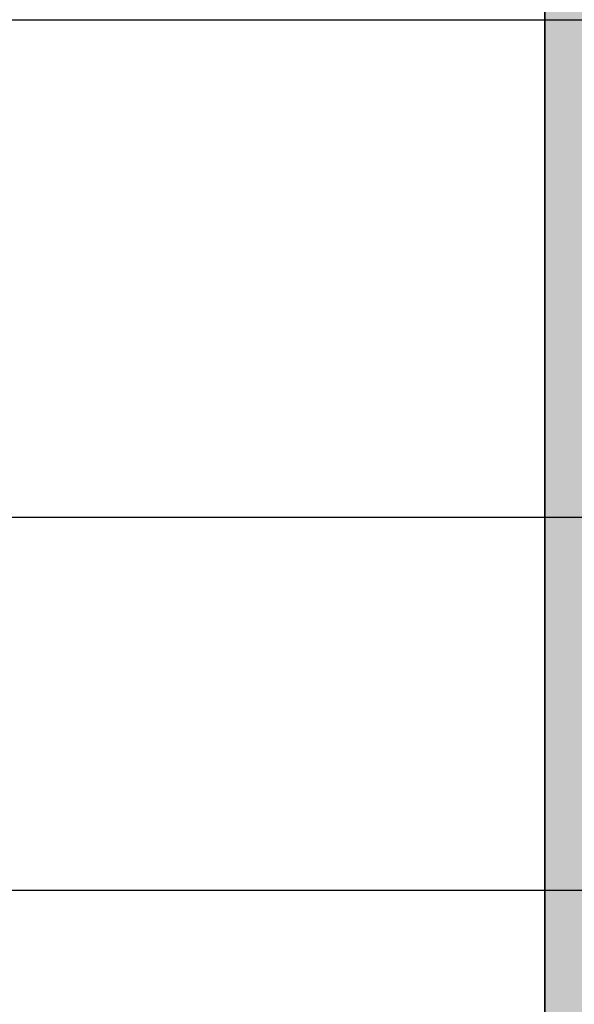
# Model space of a CAD drawing. Units: inches. Extents: x 925 to 2834, y 111 to 1355.
# Tile 20 of 25: x 1737 to 1844, y 882 to 1072. Entities that reach past the tile are written whole.
import ezdxf

# ---------------------------------------------------------------- set-up
doc = ezdxf.new("R2010")
doc.units = ezdxf.units.IN
doc.header["$MEASUREMENT"] = 0
for name, color, linetype, lineweight in [('A-ANNO-DIMS', 2, 'Continuous', 18), ('A-ANNO-TTLB', 7, 'Continuous', 35), ('A-FLOR-PATT', 252, 'Continuous', 13)]:
    doc.layers.add(name, color=color, linetype=linetype, lineweight=lineweight)
doc.styles.get("Standard").update_dxf_attribs({"font": 'arial.ttf'})
doc.dimstyles.get("Standard").update_dxf_attribs({"dimtxt": 6, "dimasz": 3, "dimexe": 0.18, "dimexo": 0.0625, "dimgap": 0.09, "dimtad": 0, "dimtih": 1, "dimtoh": 1, "dimdec": 1, "dimzin": 0, "dimdsep": 46, "dimlunit": 3, "dimtxsty": 'Standard', "dimblk": 'ARCHTICK', "dimcen": 0.09, "dimadec": 0, "dimazin": 0, "dimtfac": 1, "dimtdec": 1, "dimtofl": 0, "dimtmove": 0, "dimatfit": 3, "dimfxl": 1, "dimtolj": 1, "dimtzin": 0, "dimarcsym": 0})

# ---------------------------------------------------------------- blocks, each defined once
blk = doc.blocks.new('_ArchTick')
at = {"color": 0, "linetype": 'ByBlock', "const_width": 0.15}
blk.add_lwpolyline([(-0.5, -0.5), (0.5, 0.5)], dxfattribs=at)
blk = doc.blocks.new('*D47')
at = {"layer": 'A-ANNO-DIMS', "color": 0, "lineweight": -2, "transparency": 16777216}
for p, q in [((1708.78, 903.59), (1988.62, 903.59)), ((1988.44, 903.59), (1988.44, 869.23)), ((1988.44, 828.59), (1988.44, 862.95)), ((1708.78, 828.59), (1988.62, 828.59))]:
    blk.add_line(p, q, dxfattribs=at)
at = {"layer": 'Defpoints', "color": 0, "transparency": 16777216}
for p in [(1708.71, 903.59), (1988.44, 903.59), (1708.71, 828.59)]:
    blk.add_point(p, dxfattribs=at)
at = {"layer": 'A-ANNO-DIMS', "color": 0, "lineweight": -2, "transparency": 16777216, "xscale": 3, "yscale": 3, "zscale": 3}
for p, rotation in [((1988.44, 903.59), 90), ((1988.44, 828.59), 270)]:
    blk.add_blockref('_ArchTick', p, dxfattribs=dict(at, rotation=rotation))
at = {"layer": 'A-ANNO-DIMS', "color": 0, "transparency": 16777216, "insert": (1988.44, 866.09), "char_height": 6, "attachment_point": 5}
blk.add_mtext('\\A1;75', dxfattribs=at)
blk = doc.blocks.new('*D48')
at = {"layer": 'A-ANNO-DIMS', "color": 0, "lineweight": -2, "transparency": 16777216}
for p, q in [((1708.78, 975.59), (1988.62, 975.59)), ((1988.44, 975.59), (1988.44, 942.69)), ((1988.44, 903.59), (1988.44, 936.49)), ((1708.78, 903.59), (1988.62, 903.59))]:
    blk.add_line(p, q, dxfattribs=at)
at = {"layer": 'Defpoints', "color": 0, "transparency": 16777216}
for p in [(1708.71, 975.59), (1988.44, 975.59), (1708.71, 903.59)]:
    blk.add_point(p, dxfattribs=at)
at = {"layer": 'A-ANNO-DIMS', "color": 0, "lineweight": -2, "transparency": 16777216, "xscale": 3, "yscale": 3, "zscale": 3}
for p, rotation in [((1988.44, 975.59), 90), ((1988.44, 903.59), 270)]:
    blk.add_blockref('_ArchTick', p, dxfattribs=dict(at, rotation=rotation))
at = {"layer": 'A-ANNO-DIMS', "color": 0, "transparency": 16777216, "insert": (1988.44, 939.59), "char_height": 6, "attachment_point": 5}
blk.add_mtext('\\A1;72', dxfattribs=at)
blk = doc.blocks.new('*D49')
at = {"layer": 'A-ANNO-DIMS', "color": 0, "lineweight": -2, "transparency": 16777216}
for p, q in [((1708.78, 1071.59), (1988.62, 1071.59)), ((1988.44, 1071.59), (1988.44, 1026.74)), ((1988.44, 975.59), (1988.44, 1020.44)), ((1708.78, 975.59), (1988.62, 975.59))]:
    blk.add_line(p, q, dxfattribs=at)
at = {"layer": 'Defpoints', "color": 0, "transparency": 16777216}
for p in [(1708.71, 1071.59), (1988.44, 1071.59), (1708.71, 975.59)]:
    blk.add_point(p, dxfattribs=at)
at = {"layer": 'A-ANNO-DIMS', "color": 0, "lineweight": -2, "transparency": 16777216, "xscale": 3, "yscale": 3, "zscale": 3}
for p, rotation in [((1988.44, 1071.59), 90), ((1988.44, 975.59), 270)]:
    blk.add_blockref('_ArchTick', p, dxfattribs=dict(at, rotation=rotation))
at = {"layer": 'A-ANNO-DIMS', "color": 0, "transparency": 16777216, "insert": (1988.44, 1023.59), "char_height": 6, "attachment_point": 5}
blk.add_mtext('\\A1;96', dxfattribs=at)
blk = doc.blocks.new('*D50')
at = {"layer": 'A-ANNO-DIMS', "color": 0, "lineweight": -2, "transparency": 16777216}
for p, q in [((1718.78, 1081.59), (1988.62, 1081.59)), ((1988.44, 1081.59), (1988.44, 1079.74)), ((1988.44, 1071.59), (1988.44, 1073.44)), ((1708.78, 1071.59), (1988.62, 1071.59))]:
    blk.add_line(p, q, dxfattribs=at)
at = {"layer": 'Defpoints', "color": 0, "transparency": 16777216}
for p in [(1718.71, 1081.59), (1988.44, 1081.59), (1708.71, 1071.59)]:
    blk.add_point(p, dxfattribs=at)
at = {"layer": 'A-ANNO-DIMS', "color": 0, "lineweight": -2, "transparency": 16777216, "xscale": 3, "yscale": 3, "zscale": 3}
for p, rotation in [((1988.44, 1081.59), 90), ((1988.44, 1071.59), 270)]:
    blk.add_blockref('_ArchTick', p, dxfattribs=dict(at, rotation=rotation))
at = {"layer": 'A-ANNO-DIMS', "color": 0, "transparency": 16777216, "insert": (1988.44, 1076.59), "char_height": 6, "attachment_point": 5}
blk.add_mtext('\\A1;10', dxfattribs=at)

msp = doc.modelspace()

# ---------------------------------------------------------------- hatches: boundary and pattern name
at = {"layer": 'A-FLOR-PATT', "transparency": 33554605}
h = msp.add_hatch(color=256, dxfattribs=at)
h.dxf.hatch_style = 1
h.paths.add_polyline_path([(1931.688, 1294.5638), (991.7375, 1294.5638), (991.7375, 172.1134), (1931.688, 172.1134)])
h.paths.add_polyline_path([(1910.7128, 1273.5886), (1910.7128, 193.0886), (1012.7128, 193.0886), (1012.7128, 1273.5886)], flags=16)
h.paths.add_polyline_path([(1850.7128, 1213.5886), (1850.7128, 253.0886), (1072.7128, 253.0886), (1072.7128, 1213.5886)], flags=0)
h.paths.add_polyline_path([(1838.7128, 1201.5886), (1838.7128, 265.0886), (1084.7128, 265.0886), (1084.7128, 530.5886), (1084.7128, 1201.5886)], flags=0)
h.paths.add_polyline_path([(1547.6758, 1155.7396), (1547.6758, 1119.115), (1513.0687, 1119.115), (1513.0687, 1155.7396)], flags=0)
h.paths.add_polyline_path([(1600.1067, 1154.9439), (1634.7139, 1154.9439), (1634.7139, 1119.115), (1600.1067, 1119.115)], flags=0)
h.paths.add_polyline_path([(1505.2502, 1144.5358), (1505.2502, 1119.115), (1470.643, 1119.115), (1470.643, 1144.5358)], flags=0)
h.paths.add_polyline_path([(1559.1357, 1141.0962), (1593.7428, 1141.0962), (1593.7428, 1119.115), (1559.1357, 1119.115)], flags=0)
h.paths.add_polyline_path([(1462.8966, 1154.9439), (1462.8966, 1119.115), (1428.2895, 1119.115), (1428.2895, 1154.9439)], flags=0)
h.paths.add_polyline_path([(1642.4603, 1144.5358), (1677.0675, 1144.5358), (1677.0675, 1119.115), (1642.4603, 1119.115)], flags=0)
h.paths.add_polyline_path([(1422.3508, 1141.0962), (1422.3508, 1119.115), (1387.7436, 1119.115), (1387.7436, 1141.0962)], flags=0)
h.paths.add_polyline_path([(1684.8859, 1155.7396), (1719.4931, 1155.7396), (1719.4931, 1119.115), (1684.8859, 1119.115)], flags=0)
h.paths.add_polyline_path([(1718.7128, 1081.5886), (1718.7128, 1050.1249), (1715.7128, 1050.1249), (1715.7128, 1026.1249), (1715.7128, 1002.1249), (1718.7128, 1002.1249), (1730.7128, 1002.1249), (1730.7128, 998.1249), (1730.7128, 990.1249), (1730.7128, 986.1249), (1718.7128, 986.1249), (1718.7128, 893.5886), (1715.3735, 893.5886), (1715.3735, 891.5886), (1713.3735, 891.5886, 0.41421356), (1677.3735, 855.5886), (1713.3735, 855.5886), (1713.3735, 853.5886), (1715.3735, 853.5886), (1715.3735, 851.5886), (1718.7128, 851.5886), (1718.7128, 821.5865), (1734.4655, 821.5865), (1734.3735, 819.5886, -0.41421356), (1712.4415, 793.5886), (1712.4415, 791.5886), (1718.7128, 791.5886), (1718.7128, 717.5886), (1718.7128, 669.5886), (1732.7128, 669.5886), (1732.7128, 665.5886), (1732.7128, 641.5886), (1732.7128, 634.5886), (1732.7128, 610.5886), (1732.7128, 603.5886), (1718.7128, 603.5886), (1718.7128, 385.0886), (1434.2128, 385.0886), (1434.2128, 530.5886), (1410.2128, 530.5886), (1408.2128, 530.5886), (1408.2128, 532.5886, 0.41421356), (1372.2128, 568.5886), (1372.2128, 532.5886), (1370.2128, 532.5886), (1370.2128, 530.5886), (1368.2128, 530.5886), (1282.2128, 530.5886), (1210.2128, 530.5886), (1200.2128, 530.5886), (1200.2128, 542.1915), (1183.2307, 542.1915), (1183.2307, 546.1915), (1200.2128, 546.1915), (1200.2128, 572.1915), (1183.2307, 572.1915), (1183.2307, 576.1915), (1200.2128, 576.1915), (1200.2128, 727.5886), (1210.2128, 727.5886), (1234.2128, 727.5886), (1259.7128, 727.5886), (1259.7128, 775.5886), (1259.7128, 799.5886), (1259.7128, 847.5886), (1259.7128, 993.5872), (1259.7128, 1065.5872), (1259.7128, 1071.5886), (1219.6318, 1071.5886), (1219.6318, 1081.5886), (1084.7128, 1081.5886), (1084.7128, 1119.115), (1256.8974, 1119.115), (1256.8974, 1154.9439), (1291.5046, 1154.9439), (1291.5046, 1119.115), (1256.8974, 1119.115), (1256.6723, 1081.5886), (1293.7128, 1081.5886), (1341.7128, 1081.5886), (1341.7128, 1093.5886), (1347.7128, 1093.5886), (1371.7128, 1093.5886), (1377.7128, 1093.5886), (1377.7128, 1081.5886), (1668.7128, 1081.5886), (1668.7128, 1117.5886), (1675.7128, 1117.5886), (1711.7128, 1117.5886), (1718.7128, 1117.5886)], flags=0)
h.paths.add_polyline_path([(1376.2838, 1155.7396), (1376.2838, 1119.115), (1341.6766, 1119.115), (1341.6766, 1155.7396)], flags=0)
h.paths.add_polyline_path([(1341.7128, 1076.0886), (1293.7128, 1076.0886), (1293.7128, 1071.5886), (1269.7128, 1071.5886), (1269.7128, 1065.5872), (1266.7128, 1065.5872), (1266.7128, 1029.5872), (1265.7128, 1029.5872), (1265.7128, 993.5872), (1269.7128, 993.5872), (1269.7128, 903.5886), (1269.7128, 893.5886), (1269.7128, 847.5886), (1265.2128, 847.5886), (1265.2128, 799.5886), (1269.7128, 799.5886), (1269.7128, 775.5886), (1265.2128, 775.5886), (1265.2128, 727.5886), (1269.7128, 727.5886), (1444.2128, 727.5886), (1444.2128, 717.5886), (1234.2128, 717.5886), (1234.2128, 722.0886), (1210.2128, 722.0886), (1210.2128, 717.5886), (1210.2128, 540.5886), (1210.2128, 536.0886), (1282.2128, 536.0886), (1282.2128, 535.0886), (1210.2128, 535.0886), (1210.2128, 540.5886), (1210.2128, 717.5886), (1210.2128, 723.0886), (1234.2128, 723.0886), (1234.2128, 717.5886), (1444.2128, 717.5886), (1444.2128, 727.5886), (1269.7128, 727.5886), (1264.2128, 727.5886), (1264.2128, 775.5886), (1269.7128, 775.5886), (1269.7128, 799.5886), (1264.2128, 799.5886), (1264.2128, 847.5886), (1269.7128, 847.5886), (1269.7128, 893.5886), (1269.7128, 903.5886), (1269.7128, 993.5872), (1264.7128, 993.5872), (1264.7128, 1029.5872), (1265.7128, 1029.5872), (1265.7128, 1065.5872), (1269.7128, 1065.5872), (1269.7128, 1071.5886), (1293.7128, 1071.5886), (1293.7128, 1077.0886), (1341.7128, 1077.0886)], flags=0)
h.paths.add_polyline_path([(1730.9529, 1141.0962), (1765.5601, 1141.0962), (1765.5601, 1119.115), (1730.9529, 1119.115)], flags=0)
h.paths.add_polyline_path([(1333.8582, 1144.5358), (1333.8582, 1119.115), (1299.251, 1119.115), (1299.251, 1144.5358)], flags=0)
h.paths.add_polyline_path([(1592.7128, 968.5886), (1596.0342, 968.5886), (1602.7128, 968.5886), (1708.7128, 968.5886), (1708.7128, 903.5886), (1602.7128, 903.5886), (1602.7128, 938.5886), (1592.7128, 938.5886), (1592.7128, 903.5886), (1451.7128, 903.5886), (1451.7128, 893.5886), (1511.7128, 893.5886), (1511.7128, 881.5886), (1515.2128, 881.5886), (1518.7128, 881.5886), (1518.7128, 893.5886), (1592.7128, 893.5886), (1592.7128, 799.5886), (1518.7128, 799.5886), (1518.7128, 857.5886), (1511.7128, 857.5886), (1511.7128, 799.5886), (1511.7128, 772.0886), (1521.7128, 772.0886), (1521.7128, 792.5886), (1592.7128, 792.5886), (1592.7128, 727.5886), (1521.7128, 727.5886), (1521.7128, 748.0886), (1511.7128, 748.0886), (1511.7128, 717.5886), (1708.7128, 717.5886), (1714.2128, 717.5886), (1714.2128, 669.5886), (1708.7128, 669.5886), (1708.7128, 641.5886), (1492.2128, 641.5886), (1492.2128, 631.5886), (1621.2128, 631.5886), (1621.2128, 443.0886), (1625.7128, 443.0886), (1625.7128, 503.0886), (1625.7128, 507.5886), (1625.7128, 631.5886), (1708.7128, 631.5886), (1708.7128, 507.5886), (1655.7128, 507.5886), (1655.7128, 503.0886), (1708.7128, 503.0886), (1708.7128, 395.0886), (1625.7128, 395.0886), (1625.7128, 419.0886), (1621.2128, 419.0886), (1621.2128, 395.0886), (1482.2128, 395.0886), (1482.2128, 385.0886), (1434.2128, 385.0886), (1434.2128, 433.0886), (1444.2128, 433.0886), (1444.2128, 631.5886), (1450.2128, 631.5886), (1450.2128, 634.91), (1452.2128, 634.91), (1452.2128, 669.5886), (1454.2128, 669.5886, -0.40021217), (1490.1712, 635.3173), (1492.2128, 635.3173), (1492.2128, 641.5886), (1564.7128, 641.5886), (1564.7128, 677.5886), (1672.7128, 677.5886), (1672.7128, 681.5886), (1564.7128, 681.5886), (1564.7128, 717.5886), (1511.7128, 717.5886), (1511.7128, 748.0886), (1511.7128, 772.0886), (1511.7128, 799.5886), (1511.7128, 857.5886), (1511.8913, 857.5886), (1511.8913, 859.5886), (1515.6201, 859.5886, 0.41421356), (1537.552, 879.5886), (1513.552, 879.5886), (1511.8913, 879.5886), (1511.8913, 881.5886), (1511.7128, 881.5886), (1511.7128, 893.5886), (1451.7128, 893.5886), (1451.7128, 903.5886), (1592.7128, 903.5886), (1592.7128, 938.5886), (1592.7128, 940.5886), (1596.4415, 940.5886, 0.41421356), (1618.3735, 966.5886), (1594.3735, 966.5886), (1592.7128, 966.5886)], flags=0)
h.paths.add_polyline_path([(1377.7128, 903.5886), (1377.7128, 893.5886), (1305.7128, 893.5886), (1305.7128, 903.5886)], flags=0)
h.paths.add_polyline_path([(1708.7128, 821.5886), (1712.0342, 821.5886), (1712.0342, 819.5886), (1710.3735, 819.5886), (1708.7128, 819.5886)], flags=0)
h.paths.add_polyline_path([(1576.7128, 695.1992), (1575.5896, 693.6649), (1575.9687, 694.6994), (1575.4438, 695.1992), (1575.9687, 695.699), (1575.5896, 696.7335)], flags=0)
h.paths.add_polyline_path([(1565.9817, 662.3134), (1565.4568, 661.8136), (1565.8359, 660.7791), (1564.7128, 662.3134), (1565.8359, 663.8477), (1565.4568, 662.8132)], flags=0)
h.paths.add_polyline_path([(1444.2128, 433.0886), (1444.2128, 395.0886), (1482.2128, 395.0886), (1482.2128, 389.0886), (1438.2128, 389.0886), (1438.2128, 391.8608), (1438.2128, 433.0886)], flags=0)
h.paths.add_polyline_path([(1410.2128, 506.5886), (1410.2128, 289.0886), (1108.7128, 289.0886), (1108.7128, 506.5886)], flags=0)
h.paths.add_polyline_path([(1612.3153, 838.3016), (1680.4151, 838.3016), (1680.4151, 851.3131), (1612.3153, 851.3131)], flags=8)
h.paths.add_polyline_path([(1208.3174, 395.0436), (1282.1017, 395.0436), (1282.1017, 408.0552), (1208.3174, 408.0552)], flags=8)
h.paths.add_polyline_path([(1291.8049, 598.7427), (1369.8017, 598.7427), (1369.8017, 611.7542), (1291.8049, 611.7542)], flags=8)
h.paths.add_polyline_path([(1119.679, 917.3022), (1191.0817, 917.3022), (1191.0817, 930.3137), (1119.679, 930.3137)], flags=8)
h.paths.add_polyline_path([(1332.2261, 815.9808), (1410.2258, 815.9808), (1410.2258, 829.001), (1332.2261, 829.001)], flags=8)
h.paths.add_polyline_path([(1390.9013, 955.8158), (1475.4981, 955.8158), (1475.4981, 968.8273), (1390.9013, 968.8273)], flags=8)
h.paths.add_polyline_path([(1620.3436, 998.9325), (1688.4434, 998.9325), (1688.4434, 1011.944), (1620.3436, 1011.944)], flags=8)
h.paths.add_polyline_path([(1620.3436, 914.1039), (1691.7405, 914.1039), (1691.7405, 927.1155), (1620.3436, 927.1155)], flags=8)
h.paths.add_polyline_path([(1521.4542, 816.005), (1589.5569, 816.005), (1589.5569, 829.0253), (1521.4542, 829.0253)], flags=8)
h.paths.add_polyline_path([(1528.524, 740.3497), (1602.3082, 740.3497), (1602.3082, 753.3613), (1528.524, 753.3613)], flags=8)
h.paths.add_polyline_path([(1627.6094, 762.6128), (1702.3091, 762.6128), (1702.3091, 775.6244), (1627.6094, 775.6244)], flags=8)
h.paths.add_polyline_path([(1610.5442, 657.2751), (1684.3284, 657.2751), (1684.3284, 670.2867), (1610.5442, 670.2867)], flags=8)
h.paths.add_polyline_path([(1636.6983, 519.472), (1711.3981, 519.472), (1711.3981, 532.4835), (1636.6983, 532.4835)], flags=8)
h.paths.add_polyline_path([(1616.8577, 424.8539), (1694.8545, 424.8539), (1694.8545, 437.8654), (1616.8577, 437.8654)], flags=8)
h.paths.add_polyline_path([(1506.1456, 460.8838), (1579.9299, 460.8838), (1579.9299, 473.8953), (1506.1456, 473.8953)], flags=8)
h.paths.add_polyline_path([(1624.6119, 784.6011), (1696.9185, 784.6011), (1696.9185, 797.7864), (1624.6119, 797.7864)], flags=8)
h.paths.add_polyline_path([(1606.3732, 854.2194), (1683.3039, 854.2194), (1683.3039, 867.4048), (1606.3732, 867.4048)], flags=8)
h.paths.add_polyline_path([(1127.8008, 940.3581), (1165.1637, 940.3581), (1165.1637, 953.5348), (1127.8008, 953.5348)], flags=8)
h.paths.add_polyline_path([(1620.8657, 1019.4968), (1677.3447, 1019.4968), (1677.3447, 1032.6735), (1620.8657, 1032.6735)], flags=8)
h.paths.add_polyline_path([(1620.8643, 930.1821), (1703.0564, 930.1821), (1703.0564, 943.3675), (1620.8643, 943.3675)], flags=8)
h.paths.add_polyline_path([(1324.5702, 836.8338), (1408.0892, 836.8338), (1408.0892, 850.0191), (1324.5702, 850.0191)], flags=8)
h.paths.add_polyline_path([(1281.6584, 622.8885), (1383.6213, 622.8885), (1383.6213, 636.0739), (1281.6584, 636.0739)], flags=8)
h.paths.add_polyline_path([(1210.6721, 416.7893), (1269.1299, 416.7893), (1269.1299, 429.9747), (1210.6721, 429.9747)], flags=8)
h.paths.add_polyline_path([(1507.8264, 477.4836), (1586.7329, 477.4836), (1586.7329, 490.669), (1507.8264, 490.669)], flags=8)
h.paths.add_polyline_path([(1643.6238, 443.8135), (1696.6696, 443.8135), (1696.6696, 456.5643), (1643.6238, 456.5643)], flags=8)
h.paths.add_polyline_path([(1647.2466, 540.5638), (1693.1825, 540.5638), (1693.1825, 553.7491), (1647.2466, 553.7491)], flags=8)
h.paths.add_polyline_path([(1626.0633, 668.5064), (1673.3174, 668.5064), (1673.3174, 681.6831), (1626.0633, 681.6831)], flags=8)
h.paths.add_polyline_path([(1538.2915, 830.7872), (1567.5942, 830.7872), (1567.5942, 843.5293), (1538.2915, 843.5293)], flags=8)
h.paths.add_polyline_path([(1530.9338, 754.0477), (1559.576, 754.0477), (1559.576, 766.7898), (1530.9338, 766.7898)], flags=8)
h.paths.add_polyline_path([(1351.2461, 979.2309), (1513.8919, 979.2309), (1513.8919, 992.4076), (1351.2461, 992.4076)], flags=8)
at = {"layer": 'A-FLOR-PATT'}
h = msp.add_hatch(color=256, dxfattribs=at)
h.dxf.hatch_style = 1
h.paths.add_polyline_path([(1850.7128, 1213.5886), (1072.7128, 1213.5886), (1072.7128, 253.0886), (1850.7128, 253.0886)])
h.paths.add_polyline_path([(1084.7128, 1201.5886), (1838.7128, 1201.5886), (1838.7128, 265.0886), (1084.7128, 265.0886)], flags=16)
h.paths.add_polyline_path([(1183.2307, 576.1915), (1200.2128, 576.1915), (1200.2128, 727.5886), (1210.2128, 727.5886), (1234.2128, 727.5886), (1259.7128, 727.5886), (1259.7128, 775.5886), (1259.7128, 799.5886), (1259.7128, 847.5886), (1259.7128, 993.5872), (1259.7128, 1065.5872), (1259.7128, 1071.5886), (1219.6318, 1071.5886), (1219.6318, 1081.5886), (1293.7128, 1081.5886), (1341.7128, 1081.5886), (1341.7128, 1093.5886), (1347.7128, 1093.5886), (1347.7128, 1081.5886), (1371.7128, 1081.5886), (1371.7128, 1093.5886), (1377.7128, 1093.5886), (1377.7128, 1081.5886), (1668.7128, 1081.5886), (1668.7128, 1117.5886), (1675.7128, 1117.5886), (1675.7128, 1081.5886), (1711.7128, 1081.5886), (1711.7128, 1117.5886), (1718.7128, 1117.5886), (1718.7128, 1081.5886), (1718.7128, 1050.1249), (1715.7128, 1050.1249), (1715.7128, 1026.1249), (1715.7128, 1002.1249), (1718.7128, 1002.1249), (1730.7128, 1002.1249), (1730.7128, 998.1249), (1730.7128, 990.1249), (1730.7128, 986.1249), (1718.7128, 986.1249), (1718.7128, 893.5886), (1715.3735, 893.5886), (1715.3735, 891.5886), (1713.3735, 891.5886, 0.41421356), (1677.3735, 855.5886), (1713.3735, 855.5886), (1713.3735, 853.5886), (1715.3735, 853.5886), (1715.3735, 851.5886), (1718.7128, 851.5886), (1718.7128, 821.5865), (1734.4655, 821.5865), (1734.3735, 819.5886, -0.41421356), (1712.4415, 793.5886), (1712.4415, 791.5886), (1718.7128, 791.5886), (1718.7128, 717.5886), (1718.7128, 669.5886), (1732.7128, 669.5886), (1732.7128, 665.5886), (1732.7128, 641.5886), (1732.7128, 634.5886), (1732.7128, 610.5886), (1732.7128, 603.5886), (1718.7128, 603.5886), (1718.7128, 385.0886), (1434.2128, 385.0886), (1434.2128, 433.0886), (1434.2128, 530.5886), (1410.2128, 530.5886), (1408.2128, 530.5886), (1408.2128, 532.5886, 0.41421356), (1372.2128, 568.5886), (1372.2128, 532.5886), (1370.2128, 532.5886), (1370.2128, 530.5886), (1368.2128, 530.5886), (1282.2128, 530.5886), (1210.2128, 530.5886), (1200.2128, 530.5886), (1200.2128, 542.1915), (1183.2307, 542.1915), (1183.2307, 546.1915), (1200.2128, 546.1915), (1200.2128, 572.1915), (1183.2307, 572.1915)], flags=0)
h.paths.add_polyline_path([(1210.2128, 717.5886), (1210.2128, 723.0886), (1234.2128, 723.0886), (1234.2128, 717.5886), (1444.2128, 717.5886), (1444.2128, 727.5886), (1269.7128, 727.5886), (1264.2128, 727.5886), (1264.2128, 775.5886), (1269.7128, 775.5886), (1269.7128, 799.5886), (1264.2128, 799.5886), (1264.2128, 847.5886), (1269.7128, 847.5886), (1269.7128, 893.5886), (1269.7128, 903.5886), (1269.7128, 993.5872), (1264.7128, 993.5872), (1264.7128, 1029.5872), (1265.7128, 1029.5872), (1265.7128, 1065.5872), (1269.7128, 1065.5872), (1269.7128, 1071.5886), (1293.7128, 1071.5886), (1293.7128, 1077.0886), (1341.7128, 1077.0886), (1341.7128, 1076.0886), (1293.7128, 1076.0886), (1293.7128, 1071.5886), (1269.7128, 1071.5886), (1269.7128, 1065.5872), (1266.7128, 1065.5872), (1266.7128, 1029.5872), (1265.7128, 1029.5872), (1265.7128, 993.5872), (1269.7128, 993.5872), (1269.7128, 903.5886), (1269.7128, 893.5886), (1269.7128, 847.5886), (1265.2128, 847.5886), (1265.2128, 799.5886), (1269.7128, 799.5886), (1269.7128, 775.5886), (1265.2128, 775.5886), (1265.2128, 727.5886), (1269.7128, 727.5886), (1444.2128, 727.5886), (1444.2128, 717.5886), (1234.2128, 717.5886), (1234.2128, 722.0886), (1210.2128, 722.0886), (1210.2128, 717.5886), (1210.2128, 540.5886), (1210.2128, 536.0886), (1282.2128, 536.0886), (1282.2128, 535.0886), (1210.2128, 535.0886), (1210.2128, 540.5886)], flags=0)
h.paths.add_polyline_path([(1450.2128, 634.91), (1452.2128, 634.91), (1452.2128, 669.5886), (1454.2128, 669.5886, -0.40021217), (1490.1712, 635.3173), (1492.2128, 635.3173), (1492.2128, 641.5886), (1564.7128, 641.5886), (1564.7128, 677.5886), (1672.7128, 677.5886), (1672.7128, 681.5886), (1564.7128, 681.5886), (1564.7128, 717.5886), (1511.7128, 717.5886), (1511.7128, 748.0886), (1511.7128, 772.0886), (1511.7128, 799.5886), (1511.7128, 857.5886), (1511.8913, 857.5886), (1511.8913, 859.5886), (1515.6201, 859.5886, 0.41421356), (1537.552, 879.5886), (1513.552, 879.5886), (1511.8913, 879.5886), (1511.8913, 881.5886), (1511.7128, 881.5886), (1511.7128, 893.5886), (1451.7128, 893.5886), (1451.7128, 903.5886), (1592.7128, 903.5886), (1592.7128, 938.5886), (1592.7128, 940.5886), (1596.4415, 940.5886, 0.41421356), (1618.3735, 966.5886), (1594.3735, 966.5886), (1592.7128, 966.5886), (1592.7128, 968.5886), (1596.0342, 968.5886), (1602.7128, 968.5886), (1708.7128, 968.5886), (1708.7128, 903.5886), (1602.7128, 903.5886), (1602.7128, 938.5886), (1592.7128, 938.5886), (1592.7128, 903.5886), (1451.7128, 903.5886), (1451.7128, 893.5886), (1511.7128, 893.5886), (1511.7128, 881.5886), (1518.7128, 881.5886), (1518.7128, 893.5886), (1592.7128, 893.5886), (1592.7128, 799.5886), (1518.7128, 799.5886), (1518.7128, 857.5886), (1511.7128, 857.5886), (1511.7128, 799.5886), (1511.7128, 772.0886), (1521.7128, 772.0886), (1521.7128, 792.5886), (1592.7128, 792.5886), (1592.7128, 727.5886), (1521.7128, 727.5886), (1521.7128, 748.0886), (1511.7128, 748.0886), (1511.7128, 717.5886), (1708.7128, 717.5886), (1714.2128, 717.5886), (1714.2128, 669.5886), (1708.7128, 669.5886), (1708.7128, 641.5886), (1492.2128, 641.5886), (1492.2128, 631.5886), (1621.2128, 631.5886), (1621.2128, 443.0886), (1625.7128, 443.0886), (1625.7128, 503.0886), (1625.7128, 507.5886), (1625.7128, 631.5886), (1708.7128, 631.5886), (1708.7128, 507.5886), (1655.7128, 507.5886), (1655.7128, 503.0886), (1708.7128, 503.0886), (1708.7128, 395.0886), (1625.7128, 395.0886), (1625.7128, 419.0886), (1621.2128, 419.0886), (1621.2128, 395.0886), (1482.2128, 395.0886), (1482.2128, 389.0886), (1438.2128, 389.0886), (1438.2128, 391.8608), (1438.2128, 433.0886), (1444.2128, 433.0886), (1444.2128, 631.5886), (1450.2128, 631.5886)], flags=0)
h.paths.add_polyline_path([(1444.2128, 433.0886), (1444.2128, 395.0886), (1482.2128, 395.0886), (1482.2128, 391.0886), (1440.2128, 391.0886), (1440.2128, 391.8608), (1440.2128, 433.0886)], flags=0)
h.paths.add_polyline_path([(1305.7128, 893.5886), (1305.7128, 903.5886), (1377.7128, 903.5886), (1377.7128, 893.5886)], flags=0)
h.paths.add_polyline_path([(1564.7128, 662.3134), (1565.8359, 663.8477), (1565.4568, 662.8132), (1565.9817, 662.3134), (1565.4568, 661.8136), (1565.8359, 660.7791)], flags=0)
h.paths.add_polyline_path([(1575.4438, 695.1992), (1575.9687, 695.699), (1575.5896, 696.7335), (1576.7128, 695.1992), (1575.5896, 693.6649), (1575.9687, 694.6994)], flags=0)
h.paths.add_polyline_path([(1708.7128, 821.5886), (1712.0342, 821.5886), (1712.0342, 819.5886), (1710.3735, 819.5886), (1708.7128, 819.5886)], flags=0)

# ---------------------------------------------------------------- linework, layer by layer
at = {"layer": 'A-ANNO-TTLB'}
for p, q in [((1838.7128, 1201.5886), (1838.7128, 265.0886)), ((1838.7128, 265.0886), (1838.7128, 1081.5886))]:
    msp.add_line(p, q, dxfattribs=at)
msp.add_lwpolyline([(1084.7128, 265.0886), (1838.7128, 265.0886), (1838.7128, 1201.5886), (1084.7128, 1201.5886)], close=True, dxfattribs=at)

# ---------------------------------------------------------------- dimensions: what is measured, and where the dimension line sits
at = {"layer": 'A-ANNO-DIMS'}
for base, p1, p2, picture, middle in [((1988.438, 1081.5886), (1708.7128, 1071.5886), (1718.7128, 1081.5886), '*D50', (1988.438, 1076.5886)), ((1988.438, 1071.5886), (1708.7128, 975.5886), (1708.7128, 1071.5886), '*D49', (1988.438, 1023.5886)), ((1988.438, 975.5886), (1708.7128, 903.5886), (1708.7128, 975.5886), '*D48', (1988.438, 939.5886)), ((1988.438, 903.5886), (1708.7128, 828.5886), (1708.7128, 903.5886), '*D47', (1988.438, 866.0886))]:
    dim = msp.add_linear_dim(base=base, p1=p1, p2=p2, angle=90, dimstyle='Standard', override={"dimdec": 0, "dimlfac": 1, "dimrnd": 0, "dimzin": 0, "dimdsep": 46, "dimlunit": 2}, dxfattribs=at)
    dim.commit()
    dim.dimension.update_dxf_attribs({"geometry": picture, "text_midpoint": middle})

doc.saveas('drawing.dxf')
